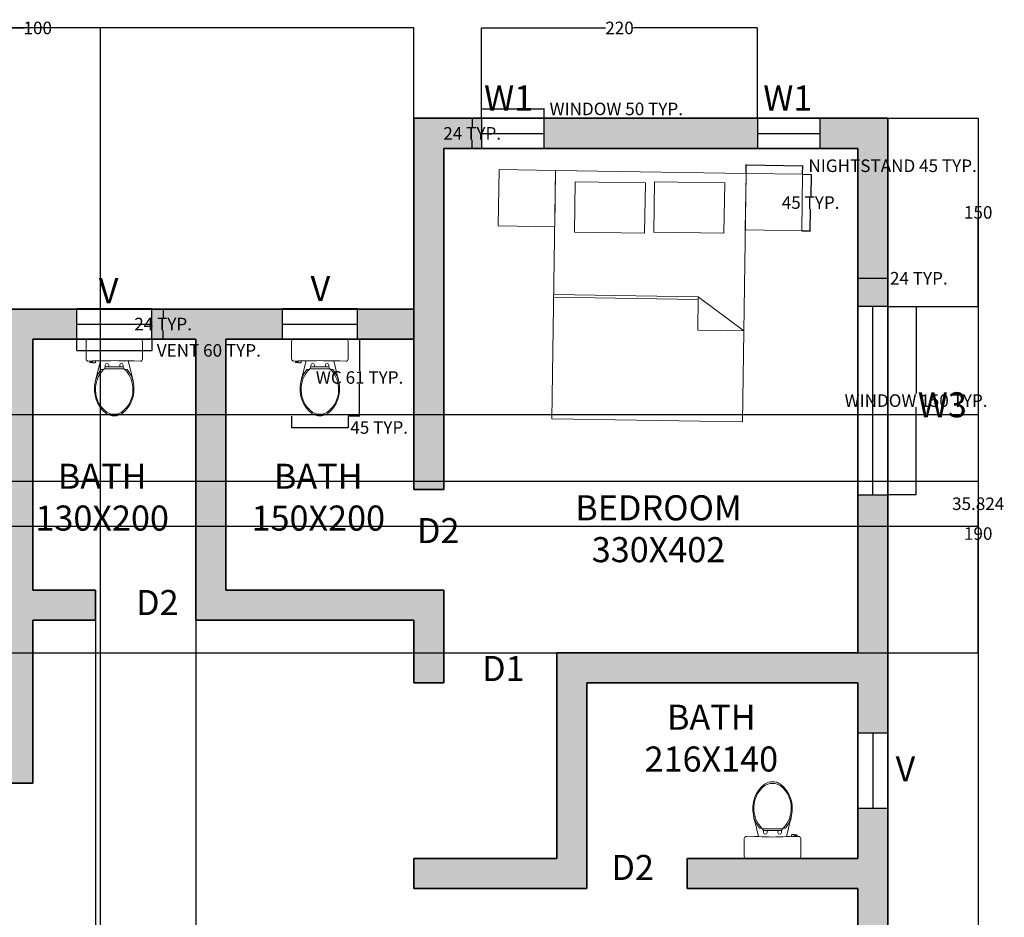
# Model space of a CAD drawing. Units: centimetres. Extents: x 1399 to 2860, y -110 to 1386.
# Tile 3 of 3: x 2074 to 2860, y 670 to 1386. Entities that reach past the tile are written whole.
import ezdxf

# ---------------------------------------------------------------- set-up
doc = ezdxf.new("R2010")
doc.units = ezdxf.units.CM
doc.header["$MEASUREMENT"] = 0
for name, color, linetype, lineweight in [('A-ANNO-DIMS', 2, 'Continuous', 18), ('A-ANNO-TEXT', 7, 'Continuous', 18), ('A-AREA-IDEN', 7, 'Continuous', 25), ('A-FLOR-FIXT', 9, 'Continuous', 18), ('A-FURN', 8, 'Continuous', 18), ('A-GLAZ', 4, 'Continuous', 25), ('A-WALL', 7, 'Continuous', 35), ('A-WALL-PATT', 252, 'Continuous', 13)]:
    doc.layers.add(name, color=color, linetype=linetype, lineweight=lineweight)
doc.styles.get("Standard").update_dxf_attribs({"font": 'arial.ttf'})
doc.dimstyles.get("Standard").update_dxf_attribs({"dimtxt": 10, "dimasz": 0.18, "dimexe": 0.18, "dimexo": 0.0625, "dimgap": 0.09, "dimtad": 0, "dimtih": 1, "dimtoh": 1, "dimdec": 4, "dimzin": 0, "dimdsep": 46, "dimtxsty": 'Standard', "dimcen": 0.09, "dimadec": 0, "dimazin": 0, "dimtfac": 1, "dimtdec": 4, "dimtofl": 0, "dimtmove": 0, "dimatfit": 3, "dimfxl": 1, "dimtolj": 1, "dimtzin": 0, "dimarcsym": 0})

# ---------------------------------------------------------------- blocks, each defined once
blk = doc.blocks.new('v')
blk.add_line((1187.13, 1404.19), (1237.13, 1404.19))
blk.add_lwpolyline([(1187.13, 1392.19), (1237.13, 1392.19), (1237.13, 1416.19), (1187.13, 1416.19)], close=True)
blk = doc.blocks.new('w1')
blk.add_line((1184.44, 1372.96), (1244.44, 1372.96))
blk.add_lwpolyline([(1184.44, 1360.96), (1244.44, 1360.96), (1244.44, 1384.96), (1184.44, 1384.96)], close=True)
blk = doc.blocks.new('w3')
blk.add_line((1235.35, 1319.41), (1085.35, 1319.41))
blk.add_lwpolyline([(1085.35, 1307.41), (1235.35, 1307.41), (1235.35, 1331.41), (1085.35, 1331.41)], close=True)
blk = doc.blocks.new('t')
for p, q in [((1419.3, 1723.8), (1428.5, 1740.5)), ((1428.5, 1740.5), (1428.5, 1758.8)), ((1461.3, 1740.5), (1428.5, 1740.5)), ((1461.3, 1758.8), (1461.3, 1740.5)), ((1513.8, 1740.5), (1461.3, 1740.5)), ((1513.8, 1740.5), (1566.3, 1740.5)), ((1566.3, 1758.8), (1566.3, 1740.5)), ((1566.3, 1740.5), (1599.1, 1740.5)), ((1599.1, 1740.5), (1599.1, 1758.8)), ((1608.3, 1723.8), (1599.1, 1740.5))]:
    blk.add_line(p, q)
for points in [[(1305.4, 1797.9), (1266, 1796.3, -0.426005), (1244, 1817.4), (1244, 1986.1, -0.414214), (1265.2, 2007.3), (1513.9, 2007.3)], [(1646.4, 1798.6, 0.00511), (1705.4, 1798.8), (1761.8, 1796.3, 0.426005), (1783.8, 1817.4), (1783.8, 1986.1, 0.414214), (1762.6, 2007.3), (1513.9, 2007.3)], [(1305.4, 1782.1), (1283.1, 1782.1, -0.3351), (1280.9, 1783.8), (1279.4, 1789.1, -0.498015), (1280.9, 1791.1), (1305.4, 1791.1)], [(1333.4, 1798.7), (1305.4, 1797.9, -0.319616)], [(1305.4, 1782.1), (1305.4, 1781.4, 0.414214), (1307.7, 1779.1), (1326.6, 1779.1, 0.414214), (1333.4, 1786), (1333.4, 1798.7)], [(1381.5, 1798.6, -0.006773), (1336.9, 1798.8), (1333.4, 1798.7, -0.55454)], [(1513.6, 1802.1, -0.010344), (1381.5, 1798.6)], [(1514.2, 1802.1, 0.010344), (1646.4, 1798.6)], [(1389.6, 1716.9, 0.114632), (1331.2, 1595.2, 0.16845)], [(1412.4, 1716.9, 0.434217), (1428.5, 1319.8, 0.182634), (1513.8, 1288.7, 2.693815)], [(1412.4, 1716.9), (1389.6, 1716.9, 0.416606)], [(1419.3, 1723.8, 0.008985), (1412.4, 1716.9, 0.182634)], [(1513.8, 1723.8), (1419.3, 1723.8, 0.008985)], [(1513.8, 1723.8), (1608.3, 1723.8, -0.444938)], [(1615.2, 1716.9, -0.434217), (1599.1, 1319.8, -0.182634), (1513.8, 1288.7, -2.693815)], [(1608.3, 1723.8, -0.008985), (1615.2, 1716.9, -0.182634)], [(1615.2, 1716.9), (1638, 1716.9, -0.416606)], [(1638, 1716.9, -0.117999), (1697.2, 1591.4, -0.16845)], [(1340.4, 1636.4, 0.005151), (1338.9, 1631, 0.024565), (1331.2, 1595.2, 0.065413)], [(1697.2, 1591.4, 0.0272), (1688.9, 1631, 0.005151), (1687.4, 1636.4, 0.103607)], [(1331.2, 1595.2, 0.288211), (1437.6, 1296.1, 0.171216), (1513.8, 1274, 2.912232)], [(1697.2, 1591.4, -0.284616), (1590, 1296.1, -0.171216), (1513.8, 1274, -2.912347)]]:
    blk.add_lwpolyline(points, format="xyb")
for points in [[(1305.4, 1797.9), (1305.4, 1791.1)], [(1305.4, 1791.1), (1305.4, 1782.1)], [(1340.4, 1636.4), (1381.5, 1798.6)], [(1687.4, 1636.4), (1646.4, 1798.6)]]:
    blk.add_lwpolyline(points)
for centre in [(1444.9, 1758.8), (1582.7, 1758.8)]:
    blk.add_arc(centre, 16.4, 0, 180)
blk = doc.blocks.new('BED')
for p, q in [((1734.14, 2886.74), (1849.51, 2886.74)), ((1734.14, 2884.74), (1849.51, 2884.74)), ((1849.51, 2886.74), (1886.14, 2860.24)), ((1886.14, 2860.24), (1849.51, 2886.74)), ((1849.51, 2886.74), (1849.51, 2860.24)), ((1849.51, 2860.24), (1886.14, 2860.24))]:
    blk.add_line(p, q)
for points in [[(1734.14, 2787.74), (1886.14, 2787.74), (1886.14, 2985.74), (1734.14, 2985.74)], [(1749.96, 2936.84), (1805.89, 2936.84), (1805.89, 2977.01), (1749.96, 2977.01)], [(1813.22, 2937.77), (1869.15, 2937.77), (1869.15, 2977.94), (1813.22, 2977.94)]]:
    blk.add_lwpolyline(points, close=True)
blk = doc.blocks.new('NIGHTSTAND-450')
blk.add_lwpolyline([(0, 45), (0, 0), (45, 0), (45, 45)], close=True)
blk = doc.blocks.new('*D13')
at = {"layer": 'A-ANNO-DIMS', "color": 0, "lineweight": -2, "transparency": 16777216}
for p, q in [((2442.8, 1307.07), (2442.8, 1314.69)), ((2442.98, 1314.51), (2492.62, 1314.51)), ((2492.8, 1307.07), (2492.8, 1314.69)), ((2492.8, 1314.51), (2492.98, 1314.51))]:
    blk.add_line(p, q, dxfattribs=at)
at = {"layer": 'A-ANNO-DIMS', "color": 0, "transparency": 16777216}
for points in [[(2442.98, 1314.54), (2442.98, 1314.48), (2442.8, 1314.51)], [(2492.62, 1314.54), (2492.62, 1314.48), (2492.8, 1314.51)]]:
    blk.add_solid(points, dxfattribs=at)
at = {"layer": 'Defpoints', "color": 0, "transparency": 16777216}
for p in [(2492.8, 1314.51), (2442.8, 1307.01), (2492.8, 1307.01)]:
    blk.add_point(p, dxfattribs=at)
at = {"layer": 'A-ANNO-DIMS', "color": 0, "transparency": 16777216, "insert": (2550.2, 1314.51), "char_height": 10, "attachment_point": 5}
blk.add_mtext('\\A1;WINDOW 50 TYP.', dxfattribs=at)
blk = doc.blocks.new('*D14')
at = {"layer": 'A-ANNO-DIMS', "color": 0, "lineweight": -2, "transparency": 16777216}
for p, q in [((2442.74, 1307.01), (2435.12, 1307.01)), ((2435.3, 1306.83), (2435.3, 1300.12)), ((2435.3, 1283.19), (2435.3, 1289.9)), ((2442.74, 1283.01), (2435.12, 1283.01))]:
    blk.add_line(p, q, dxfattribs=at)
at = {"layer": 'A-ANNO-DIMS', "color": 0, "transparency": 16777216}
for points in [[(2435.27, 1306.83), (2435.33, 1306.83), (2435.3, 1307.01)], [(2435.27, 1283.19), (2435.33, 1283.19), (2435.3, 1283.01)]]:
    blk.add_solid(points, dxfattribs=at)
at = {"layer": 'Defpoints', "color": 0, "transparency": 16777216}
for p in [(2435.3, 1307.01), (2442.8, 1307.01), (2442.8, 1283.01)]:
    blk.add_point(p, dxfattribs=at)
at = {"layer": 'A-ANNO-DIMS', "color": 0, "transparency": 16777216, "insert": (2435.3, 1295.01), "char_height": 10, "attachment_point": 5}
blk.add_mtext('\\A1;24 TYP.', dxfattribs=at)
blk = doc.blocks.new('*D15')
at = {"layer": 'A-ANNO-DIMS', "color": 0, "lineweight": -2, "transparency": 16777216}
for p, q in [((2766.86, 1157.01), (2789.48, 1157.01)), ((2789.3, 1156.83), (2789.3, 1087.27)), ((2789.3, 1007.19), (2789.3, 1076.75)), ((2766.86, 1007.01), (2789.48, 1007.01))]:
    blk.add_line(p, q, dxfattribs=at)
at = {"layer": 'A-ANNO-DIMS', "color": 0, "transparency": 16777216}
for points in [[(2789.27, 1156.83), (2789.33, 1156.83), (2789.3, 1157.01)], [(2789.27, 1007.19), (2789.33, 1007.19), (2789.3, 1007.01)]]:
    blk.add_solid(points, dxfattribs=at)
at = {"layer": 'Defpoints', "color": 0, "transparency": 16777216}
for p in [(2766.8, 1157.01), (2766.8, 1007.01), (2789.3, 1007.01)]:
    blk.add_point(p, dxfattribs=at)
at = {"layer": 'A-ANNO-DIMS', "color": 0, "transparency": 16777216, "insert": (2789.3, 1082.01), "char_height": 10, "attachment_point": 5}
blk.add_mtext('\\A1;WINDOW 150 TYP.', dxfattribs=at)
blk = doc.blocks.new('*D16')
at = {"layer": 'A-ANNO-DIMS', "color": 0, "lineweight": -2, "transparency": 16777216}
for p, q in [((2742.8, 1157.07), (2742.8, 1179.69)), ((2742.98, 1179.51), (2766.62, 1179.51)), ((2766.8, 1157.07), (2766.8, 1179.69)), ((2766.8, 1179.51), (2766.98, 1179.51))]:
    blk.add_line(p, q, dxfattribs=at)
at = {"layer": 'A-ANNO-DIMS', "color": 0, "transparency": 16777216}
for points in [[(2742.98, 1179.54), (2742.98, 1179.48), (2742.8, 1179.51)], [(2766.62, 1179.54), (2766.62, 1179.48), (2766.8, 1179.51)]]:
    blk.add_solid(points, dxfattribs=at)
at = {"layer": 'Defpoints', "color": 0, "transparency": 16777216}
for p in [(2766.8, 1179.51), (2742.8, 1157.01), (2766.8, 1157.01)]:
    blk.add_point(p, dxfattribs=at)
at = {"layer": 'A-ANNO-DIMS', "color": 0, "transparency": 16777216, "insert": (2791.5, 1179.51), "char_height": 10, "attachment_point": 5}
blk.add_mtext('\\A1;24 TYP.', dxfattribs=at)
blk = doc.blocks.new('*D17')
at = {"layer": 'A-ANNO-DIMS', "color": 0, "lineweight": -2, "transparency": 16777216}
for p, q in [((2119.8, 1130.95), (2119.8, 1121.83)), ((2179.8, 1130.95), (2179.8, 1121.83)), ((2119.98, 1122.01), (2179.62, 1122.01)), ((2179.8, 1122.01), (2179.98, 1122.01))]:
    blk.add_line(p, q, dxfattribs=at)
at = {"layer": 'A-ANNO-DIMS', "color": 0, "transparency": 16777216}
for points in [[(2119.98, 1122.04), (2119.98, 1121.98), (2119.8, 1122.01)], [(2179.62, 1122.04), (2179.62, 1121.98), (2179.8, 1122.01)]]:
    blk.add_solid(points, dxfattribs=at)
at = {"layer": 'Defpoints', "color": 0, "transparency": 16777216}
for p in [(2119.8, 1131.01), (2179.8, 1131.01), (2179.8, 1122.01)]:
    blk.add_point(p, dxfattribs=at)
at = {"layer": 'A-ANNO-DIMS', "color": 0, "transparency": 16777216, "insert": (2225.24, 1122.01), "char_height": 10, "attachment_point": 5}
blk.add_mtext('\\A1;VENT 60 TYP.', dxfattribs=at)
blk = doc.blocks.new('*D18')
at = {"layer": 'A-ANNO-DIMS', "color": 0, "lineweight": -2, "transparency": 16777216}
for p, q in [((2179.86, 1155.01), (2188.98, 1155.01)), ((2188.8, 1154.83), (2188.8, 1148.12)), ((2179.86, 1131.01), (2188.98, 1131.01)), ((2188.8, 1131.19), (2188.8, 1137.9))]:
    blk.add_line(p, q, dxfattribs=at)
at = {"layer": 'A-ANNO-DIMS', "color": 0, "transparency": 16777216}
for points in [[(2188.77, 1154.83), (2188.83, 1154.83), (2188.8, 1155.01)], [(2188.77, 1131.19), (2188.83, 1131.19), (2188.8, 1131.01)]]:
    blk.add_solid(points, dxfattribs=at)
at = {"layer": 'Defpoints', "color": 0, "transparency": 16777216}
for p in [(2179.8, 1155.01), (2188.8, 1155.01), (2179.8, 1131.01)]:
    blk.add_point(p, dxfattribs=at)
at = {"layer": 'A-ANNO-DIMS', "color": 0, "transparency": 16777216, "insert": (2188.8, 1143.01), "char_height": 10, "attachment_point": 5}
blk.add_mtext('\\A1;24 TYP.', dxfattribs=at)
blk = doc.blocks.new('*D25')
at = {"layer": 'A-ANNO-DIMS', "color": 0, "lineweight": -2, "transparency": 16777216}
for p, q in [((2653.79, 1263.2), (2653.9, 1270.07)), ((2654.08, 1269.88), (2698.71, 1269.2)), ((2698.79, 1262.51), (2698.89, 1269.37)), ((2698.89, 1269.19), (2699.07, 1269.19))]:
    blk.add_line(p, q, dxfattribs=at)
at = {"layer": 'A-ANNO-DIMS', "color": 0, "transparency": 16777216}
for points in [[(2654.08, 1269.91), (2654.08, 1269.85), (2653.9, 1269.89)], [(2698.71, 1269.23), (2698.71, 1269.17), (2698.89, 1269.19)]]:
    blk.add_solid(points, dxfattribs=at)
at = {"layer": 'Defpoints', "color": 0, "transparency": 16777216}
for p in [(2698.89, 1269.19), (2653.79, 1263.14), (2698.79, 1262.44)]:
    blk.add_point(p, dxfattribs=at)
at = {"layer": 'A-ANNO-DIMS', "color": 0, "transparency": 16777216, "insert": (2770.6, 1269.19), "char_height": 10, "attachment_point": 5}
blk.add_mtext('\\A1;NIGHTSTAND 45 TYP.', dxfattribs=at)
blk = doc.blocks.new('*D26')
at = {"layer": 'A-ANNO-DIMS', "color": 0, "lineweight": -2, "transparency": 16777216}
for p, q in [((2698.85, 1262.44), (2705.72, 1262.34)), ((2705.53, 1262.16), (2705.27, 1245.02)), ((2704.85, 1217.53), (2705.11, 1234.67)), ((2698.16, 1217.45), (2705.02, 1217.34))]:
    blk.add_line(p, q, dxfattribs=at)
at = {"layer": 'A-ANNO-DIMS', "color": 0, "transparency": 16777216}
for points in [[(2705.5, 1262.16), (2705.56, 1262.16), (2705.54, 1262.34)], [(2704.82, 1217.53), (2704.88, 1217.53), (2704.84, 1217.35)]]:
    blk.add_solid(points, dxfattribs=at)
at = {"layer": 'Defpoints', "color": 0, "transparency": 16777216}
for p in [(2698.79, 1262.44), (2698.1, 1217.45), (2704.84, 1217.35)]:
    blk.add_point(p, dxfattribs=at)
at = {"layer": 'A-ANNO-DIMS', "color": 0, "transparency": 16777216, "insert": (2705.19, 1239.84), "char_height": 10, "attachment_point": 5}
blk.add_mtext('\\A1;45 TYP.', dxfattribs=at)
blk = doc.blocks.new('*D27')
at = {"layer": 'A-ANNO-DIMS', "color": 0, "lineweight": -2, "transparency": 16777216}
for p, q in [((2336.36, 1131.01), (2345.66, 1131.01)), ((2345.48, 1130.83), (2345.48, 1105.65)), ((2345.48, 1069.96), (2345.48, 1095.13)), ((2336.36, 1069.78), (2345.66, 1069.78))]:
    blk.add_line(p, q, dxfattribs=at)
at = {"layer": 'A-ANNO-DIMS', "color": 0, "transparency": 16777216}
for points in [[(2345.45, 1130.83), (2345.51, 1130.83), (2345.48, 1131.01)], [(2345.45, 1069.96), (2345.51, 1069.96), (2345.48, 1069.78)]]:
    blk.add_solid(points, dxfattribs=at)
at = {"layer": 'Defpoints', "color": 0, "transparency": 16777216}
for p in [(2336.29, 1131.01), (2345.48, 1131.01), (2336.29, 1069.78)]:
    blk.add_point(p, dxfattribs=at)
at = {"layer": 'A-ANNO-DIMS', "color": 0, "transparency": 16777216, "insert": (2345.48, 1100.39), "char_height": 10, "attachment_point": 5}
blk.add_mtext('\\A1;WC 61 TYP.', dxfattribs=at)
blk = doc.blocks.new('*D28')
at = {"layer": 'A-ANNO-DIMS', "color": 0, "lineweight": -2, "transparency": 16777216}
for p, q in [((2291.31, 1069.71), (2291.31, 1060.41)), ((2336.29, 1069.71), (2336.29, 1060.41)), ((2291.49, 1060.59), (2336.11, 1060.59)), ((2336.29, 1060.59), (2336.47, 1060.59))]:
    blk.add_line(p, q, dxfattribs=at)
at = {"layer": 'A-ANNO-DIMS', "color": 0, "transparency": 16777216}
for points in [[(2291.49, 1060.62), (2291.49, 1060.56), (2291.31, 1060.59)], [(2336.11, 1060.62), (2336.11, 1060.56), (2336.29, 1060.59)]]:
    blk.add_solid(points, dxfattribs=at)
at = {"layer": 'Defpoints', "color": 0, "transparency": 16777216}
for p in [(2291.31, 1069.78), (2336.29, 1069.78), (2336.29, 1060.59)]:
    blk.add_point(p, dxfattribs=at)
at = {"layer": 'A-ANNO-DIMS', "color": 0, "transparency": 16777216, "insert": (2361.1, 1060.59), "char_height": 10, "attachment_point": 5}
blk.add_mtext('\\A1;45 TYP.', dxfattribs=at)
blk = doc.blocks.new('*D37')
at = {"layer": 'A-ANNO-DIMS', "color": 0, "lineweight": -2, "transparency": 16777216}
for p, q in [((1482.8, 800.95), (1482.8, -103.22)), ((2766.8, -31.05), (2766.8, -103.22)), ((1482.98, -103.04), (2110.27, -103.04)), ((2766.62, -103.04), (2139.33, -103.04))]:
    blk.add_line(p, q, dxfattribs=at)
at = {"layer": 'A-ANNO-DIMS', "color": 0, "transparency": 16777216}
for points in [[(1482.98, -103.01), (1482.98, -103.07), (1482.8, -103.04)], [(2766.62, -103.01), (2766.62, -103.07), (2766.8, -103.04)]]:
    blk.add_solid(points, dxfattribs=at)
at = {"layer": 'Defpoints', "color": 0, "transparency": 16777216}
for p in [(1482.8, 801.01), (2766.8, -30.99), (2766.8, -103.04)]:
    blk.add_point(p, dxfattribs=at)
at = {"layer": 'A-ANNO-DIMS', "color": 0, "transparency": 16777216, "insert": (2124.8, -103.04), "char_height": 10, "attachment_point": 5}
blk.add_mtext('\\A1;1284', dxfattribs=at)
blk = doc.blocks.new('*D38')
at = {"layer": 'A-ANNO-DIMS', "color": 0, "lineweight": -2, "transparency": 16777216}
for p, q in [((2766.86, 1307.01), (2839.03, 1307.01)), ((2838.85, 1306.83), (2838.85, 643.21)), ((2838.85, -30.81), (2838.85, 632.81)), ((2766.86, -30.99), (2839.03, -30.99))]:
    blk.add_line(p, q, dxfattribs=at)
at = {"layer": 'A-ANNO-DIMS', "color": 0, "transparency": 16777216}
for points in [[(2838.82, 1306.83), (2838.88, 1306.83), (2838.85, 1307.01)], [(2838.82, -30.81), (2838.88, -30.81), (2838.85, -30.99)]]:
    blk.add_solid(points, dxfattribs=at)
at = {"layer": 'Defpoints', "color": 0, "transparency": 16777216}
for p in [(2766.8, 1307.01), (2838.85, 1307.01), (2766.8, -30.99)]:
    blk.add_point(p, dxfattribs=at)
at = {"layer": 'A-ANNO-DIMS', "color": 0, "transparency": 16777216, "insert": (2838.85, 638.01), "char_height": 10, "attachment_point": 5}
blk.add_mtext('\\A1;1338', dxfattribs=at)
blk = doc.blocks.new('*D39')
at = {"layer": 'A-ANNO-DIMS', "color": 0, "lineweight": -2, "transparency": 16777216}
for p, q in [((1532.8, 1155.07), (1532.8, 1379.24)), ((1532.98, 1379.06), (1949.66, 1379.06)), ((2388.62, 1379.06), (1971.94, 1379.06)), ((2388.8, 1155.07), (2388.8, 1379.24))]:
    blk.add_line(p, q, dxfattribs=at)
at = {"layer": 'A-ANNO-DIMS', "color": 0, "transparency": 16777216}
for points in [[(1532.98, 1379.09), (1532.98, 1379.03), (1532.8, 1379.06)], [(2388.62, 1379.09), (2388.62, 1379.03), (2388.8, 1379.06)]]:
    blk.add_solid(points, dxfattribs=at)
at = {"layer": 'Defpoints', "color": 0, "transparency": 16777216}
for p in [(2388.8, 1379.06), (1532.8, 1155.01), (2388.8, 1155.01)]:
    blk.add_point(p, dxfattribs=at)
at = {"layer": 'A-ANNO-DIMS', "color": 0, "transparency": 16777216, "insert": (1960.8, 1379.06), "char_height": 10, "attachment_point": 5}
blk.add_mtext('\\A1;856', dxfattribs=at)
blk = doc.blocks.new('*D44')
at = {"layer": 'A-ANNO-DIMS', "color": 0, "lineweight": -2, "transparency": 16777216}
for p, q in [((2134.8, 906.95), (2134.8, -103.22)), ((2214.8, 906.95), (2214.8, -103.22)), ((2134.98, -103.04), (2167.56, -103.04)), ((2214.62, -103.04), (2182.04, -103.04))]:
    blk.add_line(p, q, dxfattribs=at)
at = {"layer": 'A-ANNO-DIMS', "color": 0, "transparency": 16777216}
for points in [[(2134.98, -103.01), (2134.98, -103.07), (2134.8, -103.04)], [(2214.62, -103.01), (2214.62, -103.07), (2214.8, -103.04)]]:
    blk.add_solid(points, dxfattribs=at)
at = {"layer": 'Defpoints', "color": 0, "transparency": 16777216}
for p in [(2134.8, 907.01), (2214.8, 907.01), (2214.8, -103.04)]:
    blk.add_point(p, dxfattribs=at)
at = {"layer": 'A-ANNO-DIMS', "color": 0, "transparency": 16777216, "insert": (2174.8, -103.04), "char_height": 10, "attachment_point": 5}
blk.add_mtext('\\A1;80', dxfattribs=at)
blk = doc.blocks.new('*D45')
at = {"layer": 'A-ANNO-DIMS', "color": 0, "lineweight": -2, "transparency": 16777216}
for p, q in [((2038.8, 33.07), (2038.8, 1379.24)), ((2038.98, 1379.06), (2078.15, 1379.06)), ((2138.62, 1379.06), (2099.45, 1379.06)), ((2138.8, 183.07), (2138.8, 1379.24))]:
    blk.add_line(p, q, dxfattribs=at)
at = {"layer": 'A-ANNO-DIMS', "color": 0, "transparency": 16777216}
for points in [[(2038.98, 1379.09), (2038.98, 1379.03), (2038.8, 1379.06)], [(2138.62, 1379.09), (2138.62, 1379.03), (2138.8, 1379.06)]]:
    blk.add_solid(points, dxfattribs=at)
at = {"layer": 'Defpoints', "color": 0, "transparency": 16777216}
for p in [(2038.8, 1379.06), (2138.8, 183.01), (2038.8, 33.01)]:
    blk.add_point(p, dxfattribs=at)
at = {"layer": 'A-ANNO-DIMS', "color": 0, "transparency": 16777216, "insert": (2088.8, 1379.06), "char_height": 10, "attachment_point": 5}
blk.add_mtext('\\A1;100', dxfattribs=at)
blk = doc.blocks.new('*D46')
at = {"layer": 'A-ANNO-DIMS', "color": 0, "lineweight": -2, "transparency": 16777216}
for p, q in [((2442.8, 1307.07), (2442.8, 1379.24)), ((2442.98, 1379.06), (2541.6, 1379.06)), ((2662.62, 1379.06), (2564.01, 1379.06)), ((2662.8, 1307.07), (2662.8, 1379.24))]:
    blk.add_line(p, q, dxfattribs=at)
at = {"layer": 'A-ANNO-DIMS', "color": 0, "transparency": 16777216}
for points in [[(2442.98, 1379.09), (2442.98, 1379.03), (2442.8, 1379.06)], [(2662.62, 1379.09), (2662.62, 1379.03), (2662.8, 1379.06)]]:
    blk.add_solid(points, dxfattribs=at)
at = {"layer": 'Defpoints', "color": 0, "transparency": 16777216}
for p in [(2662.8, 1379.06), (2442.8, 1307.01), (2662.8, 1307.01)]:
    blk.add_point(p, dxfattribs=at)
at = {"layer": 'A-ANNO-DIMS', "color": 0, "transparency": 16777216, "insert": (2552.8, 1379.06), "char_height": 10, "attachment_point": 5}
blk.add_mtext('\\A1;220', dxfattribs=at)
blk = doc.blocks.new('*D47')
at = {"layer": 'A-ANNO-DIMS', "color": 0, "lineweight": -2, "transparency": 16777216}
for p, q in [((2766.86, 1307.01), (2839.03, 1307.01)), ((2838.85, 1306.83), (2838.85, 1237.21)), ((2838.85, 1157.19), (2838.85, 1226.81)), ((2766.86, 1157.01), (2839.03, 1157.01))]:
    blk.add_line(p, q, dxfattribs=at)
at = {"layer": 'A-ANNO-DIMS', "color": 0, "transparency": 16777216}
for points in [[(2838.82, 1306.83), (2838.88, 1306.83), (2838.85, 1307.01)], [(2838.82, 1157.19), (2838.88, 1157.19), (2838.85, 1157.01)]]:
    blk.add_solid(points, dxfattribs=at)
at = {"layer": 'Defpoints', "color": 0, "transparency": 16777216}
for p in [(2766.8, 1307.01), (2838.85, 1307.01), (2766.8, 1157.01)]:
    blk.add_point(p, dxfattribs=at)
at = {"layer": 'A-ANNO-DIMS', "color": 0, "transparency": 16777216, "insert": (2838.85, 1232.01), "char_height": 10, "attachment_point": 5}
blk.add_mtext('\\A1;150', dxfattribs=at)
blk = doc.blocks.new('*D51')
at = {"layer": 'A-ANNO-DIMS', "color": 0, "lineweight": -2, "transparency": 16777216}
for p, q in [((1600.97, 1017.69), (2839.03, 1017.69)), ((2838.85, 1017.51), (2838.85, 1004.98)), ((2838.85, 982.05), (2838.85, 994.58)), ((1600.97, 981.87), (2839.03, 981.87))]:
    blk.add_line(p, q, dxfattribs=at)
at = {"layer": 'A-ANNO-DIMS', "color": 0, "transparency": 16777216}
for points in [[(2838.82, 1017.51), (2838.88, 1017.51), (2838.85, 1017.69)], [(2838.82, 982.05), (2838.88, 982.05), (2838.85, 981.87)]]:
    blk.add_solid(points, dxfattribs=at)
at = {"layer": 'Defpoints', "color": 0, "transparency": 16777216}
for p in [(1600.91, 1017.69), (1600.91, 981.87), (2838.85, 981.87)]:
    blk.add_point(p, dxfattribs=at)
at = {"layer": 'A-ANNO-DIMS', "color": 0, "transparency": 16777216, "insert": (2838.85, 999.78), "char_height": 10, "attachment_point": 5}
blk.add_mtext('\\A1;35.824', dxfattribs=at)
blk = doc.blocks.new('*D53')
at = {"layer": 'A-ANNO-DIMS', "color": 0, "lineweight": -2, "transparency": 16777216}
for p, q in [((1790.86, 1071.01), (2839.03, 1071.01)), ((2838.85, 1070.83), (2838.85, 981.21)), ((2838.85, 881.19), (2838.85, 970.81)), ((1790.86, 881.01), (2839.03, 881.01))]:
    blk.add_line(p, q, dxfattribs=at)
at = {"layer": 'A-ANNO-DIMS', "color": 0, "transparency": 16777216}
for points in [[(2838.82, 1070.83), (2838.88, 1070.83), (2838.85, 1071.01)], [(2838.82, 881.19), (2838.88, 881.19), (2838.85, 881.01)]]:
    blk.add_solid(points, dxfattribs=at)
at = {"layer": 'Defpoints', "color": 0, "transparency": 16777216}
for p in [(1790.8, 1071.01), (2838.85, 1071.01), (1790.8, 881.01)]:
    blk.add_point(p, dxfattribs=at)
at = {"layer": 'A-ANNO-DIMS', "color": 0, "transparency": 16777216, "insert": (2838.85, 976.01), "char_height": 10, "attachment_point": 5}
blk.add_mtext('\\A1;190', dxfattribs=at)

msp = doc.modelspace()

# ---------------------------------------------------------------- hatches: boundary and pattern name
at = {"layer": 'A-WALL-PATT'}
h = msp.add_hatch(color=256, dxfattribs=at)
h.dxf.hatch_style = 1
h.paths.add_polyline_path([(1581.8022, 1155.0098), (1532.8022, 1155.0098), (1532.8022, 1081.0098), (1556.8022, 1081.0098), (1556.8022, 1131.0098), (1581.8022, 1131.0098)])
h.paths.add_polyline_path([(1556.8022, 931.0098), (1532.8022, 931.0098), (1532.8022, 881.0098), (1556.8022, 881.0098)])
h.paths.add_polyline_path([(1820.8022, 1155.0098), (1681.8022, 1155.0098), (1681.8022, 1131.0098), (1706.8022, 1131.0098), (1706.8022, 881.0098), (1730.8022, 881.0098), (1730.8022, 1131.0098), (1820.8022, 1131.0098)])
h.paths.add_polyline_path([(2119.8022, 1155.0098), (1970.8022, 1155.0098), (1970.8022, 1131.0098), (2060.8022, 1131.0098), (2060.8022, 777.0098), (2084.8022, 777.0098), (2084.8022, 907.0098), (2134.8022, 907.0098), (2134.8022, 931.0098), (2084.8022, 931.0098), (2084.8022, 1131.0098), (2119.8022, 1131.0098)])
h.paths.add_polyline_path([(2283.8022, 1155.0098), (2179.8022, 1155.0098), (2179.8022, 1131.0098), (2214.8022, 1131.0098), (2214.8022, 907.0098), (2388.8022, 907.0098), (2388.8022, 857.0098), (2412.8022, 857.0098), (2412.8022, 931.0098), (2238.8022, 931.0098), (2238.8022, 1131.0098), (2283.8022, 1131.0098)])
h.paths.add_polyline_path([(2388.8022, 1155.0098), (2343.8022, 1155.0098), (2343.8022, 1131.0098), (2388.8022, 1131.0098)], flags=17)
h.paths.add_polyline_path([(2412.8022, 1283.0098), (2442.8022, 1283.0098), (2442.8022, 1307.0098), (2388.8022, 1307.0098), (2388.8022, 1011.0098), (2412.8022, 1011.0098)])
h.paths.add_polyline_path([(2662.8022, 1307.0098), (2492.8022, 1307.0098), (2492.8022, 1283.0098), (2662.8022, 1283.0098)])
h.paths.add_polyline_path([(2766.8022, 1307.0098), (2712.8022, 1307.0098), (2712.8022, 1283.0098), (2742.8022, 1283.0098), (2742.8022, 1157.0098), (2766.8022, 1157.0098)])
h.paths.add_polyline_path([(2766.8022, 1007.0098), (2742.8022, 1007.0098), (2742.8022, 881.0098), (2502.8022, 881.0098), (2502.8022, 717.0098), (2388.8022, 717.0098), (2388.8022, 693.0098), (2526.8022, 693.0098), (2526.8022, 857.0098), (2742.8022, 857.0098), (2742.8022, 817.0098), (2766.8022, 817.0098)])
h.paths.add_polyline_path([(2766.8022, 757.0098), (2742.8022, 757.0098), (2742.8022, 717.0098), (2606.8022, 717.0098), (2606.8022, 693.0098), (2742.8022, 693.0098), (2742.8022, 598.0098), (2766.8022, 598.0098)])
h.paths.add_polyline_path([(2442.8022, 353.0098), (2412.8022, 353.0098), (2412.8022, 603.0098), (2238.8022, 603.0098), (2238.8022, 579.0098), (2388.8022, 579.0098), (2388.8022, 512.2445, -0.02916898), (2388.8858, 510.8126), (2388.8858, 458.2748), (2388.8022, 458.2748), (2388.8022, 402.9002), (2388.8024, 402.776), (2388.8858, 402.776), (2388.8858, 350.2798, -0.02916898), (2388.8022, 348.8479), (2388.8022, 329.0098), (2442.8022, 329.0098)])
h.paths.add_polyline_path([(2662.8022, 353.0098), (2492.8022, 353.0098), (2492.8022, 329.0098), (2662.8022, 329.0098)])
h.paths.add_polyline_path([(2412.8022, 329.0098), (2388.8022, 329.0098), (2388.8022, 159.0098), (2412.8022, 159.0098)])
h.paths.add_polyline_path([(2388.8022, 183.0098), (2338.8022, 183.0098), (2338.8022, 159.0098), (2388.8022, 159.0098)])
h.paths.add_polyline_path([(2188.8022, 183.0098), (2138.8022, 183.0098), (2138.8022, 159.0098), (2188.8022, 159.0098)])
h.paths.add_polyline_path([(2038.8022, 417.0098), (2014.8022, 417.0098), (2014.8022, 33.0098), (1924.8022, 33.0098), (1924.8022, 9.0098), (2038.8022, 9.0098)])
h.paths.add_polyline_path([(1774.8022, 33.0098), (1684.8022, 33.0098), (1684.8022, 63.0098), (1660.8022, 63.0098), (1660.8022, 9.0098), (1774.8022, 9.0098)])
h.paths.add_polyline_path([(1684.8022, 313.0098), (1660.8022, 313.0098), (1660.8022, 113.0098), (1684.8022, 113.0098)])
h.paths.add_polyline_path([(1924.8022, 417.0098), (1684.8022, 417.0098), (1684.8022, 497.0098), (1660.8022, 497.0098), (1660.8022, 363.0098), (1684.8022, 363.0098), (1684.8022, 393.0098), (1924.8022, 393.0098)])
h.paths.add_polyline_path([(1684.8022, 777.0098), (1660.8022, 777.0098), (1660.8022, 697.0098), (1684.8022, 697.0098)])
h.paths.add_polyline_path([(1970.8022, 801.0098), (1532.8022, 801.0098), (1532.8022, 777.0098), (1970.8022, 777.0098)])

# ---------------------------------------------------------------- linework, layer by layer
at = {"layer": 'A-WALL'}
for p, q in [((2388.8022, 1307.0098), (2766.8022, 1307.0098)), ((2388.8022, 1011.0098), (2388.8022, 1307.0098)), ((2766.8022, -30.9902), (2766.8022, 1307.0098)), ((2412.8022, 1283.0098), (2742.8022, 1283.0098)), ((2412.8022, 1011.0098), (2412.8022, 1283.0098)), ((2742.8022, 881.0098), (2742.8022, 1283.0098)), ((1532.8022, 1155.0098), (2388.8022, 1155.0098)), ((2084.8022, 1131.0098), (2214.8022, 1131.0098)), ((2084.8022, 931.0098), (2084.8022, 1131.0098)), ((2214.8022, 907.0098), (2214.8022, 1131.0098)), ((2238.8022, 931.0098), (2238.8022, 1131.0098)), ((2238.8022, 1131.0098), (2388.8022, 1131.0098)), ((2388.8022, 1011.0098), (2412.8022, 1011.0098)), ((2084.8022, 931.0098), (2134.8022, 931.0098)), ((2134.8022, 907.0098), (2134.8022, 931.0098)), ((2238.8022, 931.0098), (2412.8022, 931.0098)), ((2412.8022, 857.0098), (2412.8022, 931.0098)), ((2084.8022, 777.0098), (2084.8022, 907.0098)), ((2084.8022, 907.0098), (2134.8022, 907.0098)), ((2214.8022, 907.0098), (2388.8022, 907.0098)), ((2388.8022, 857.0098), (2388.8022, 907.0098)), ((2502.8022, 717.0098), (2502.8022, 881.0098)), ((2502.8022, 881.0098), (2742.8022, 881.0098)), ((2388.8022, 857.0098), (2412.8022, 857.0098)), ((2526.8022, 693.0098), (2526.8022, 857.0098)), ((2526.8022, 857.0098), (2742.8022, 857.0098)), ((2742.8022, 717.0098), (2742.8022, 857.0098)), ((2060.8022, 777.0098), (2084.8022, 777.0098)), ((2388.8022, 717.0098), (2502.8022, 717.0098)), ((2388.8022, 693.0098), (2388.8022, 717.0098)), ((2606.8022, 693.0098), (2606.8022, 717.0098)), ((2606.8022, 717.0098), (2742.8022, 717.0098)), ((2388.8022, 693.0098), (2526.8022, 693.0098)), ((2606.8022, 693.0098), (2742.8022, 693.0098)), ((2742.8022, 353.0098), (2742.8022, 693.0098))]:
    msp.add_line(p, q, dxfattribs=at)

# ---------------------------------------------------------------- block references
at = {"layer": 'A-FLOR-FIXT', "xscale": 0.0833333333333333, "yscale": 0.0833333333333333, "zscale": 0.0833333333333333}
for p in [(2023.6429, 963.7375), (2187.6429, 963.7375)]:
    msp.add_blockref('t', p, dxfattribs=at)
at = {"layer": 'A-FLOR-FIXT', "xscale": 0.0833333333333333, "yscale": 0.0833333333333333, "zscale": 0.0833333333333333, "rotation": 180}
msp.add_blockref('t', (2800.9615, 884.282), dxfattribs=at)
at = {"layer": 'A-FURN'}
for name, p, rotation in [('NIGHTSTAND-450', (2456.8165, 1266.17), 269.1178617061952), ('BED', (721.9098, -1693.2097), 359.1178617061952), ('NIGHTSTAND-450', (2653.7932, 1263.1371), 269.1178617061952)]:
    msp.add_blockref(name, p, dxfattribs=dict(at, rotation=rotation))
at = {"layer": 'A-GLAZ'}
for name, p in [('v', (1255.672, -109.1797)), ('v', (1475.672, -109.1797)), ('w1', (935.3655, -229.9466)), ('w1', (1099.3655, -229.9466))]:
    msp.add_blockref(name, p, dxfattribs=at)
at = {"layer": 'A-GLAZ', "rotation": 270}
for name, p in [('w3', (1435.392, 2242.3567)), ('w1', (1381.8458, 2001.4465))]:
    msp.add_blockref(name, p, dxfattribs=at)

# ---------------------------------------------------------------- texts
at = {"layer": 'A-ANNO-TEXT', "char_height": 20, "attachment_point": 1}
for s, width, insert in [('W1', 163.588182, (2444.7907, 1333.1968)), ('W1', 163.588182, (2667.4449, 1333.1968)), ('V', 163.588182, (2137.4692, 1179.6364)), ('V', 163.588182, (2306.3723, 1181.308)), ('W3', 163.588182, (2790.6959, 1088.6513)), ('D2', 163.588182, (2391.2723, 988.3825)), ('D2', 163.588182, (2167.2367, 931.0308)), ('D1', 103.726959, (2443.1948, 878.4317)), ('V', 163.588182, (2772.9464, 798.5152)), ('D2', 163.588182, (2546.3314, 719.8123))]:
    msp.add_mtext_dynamic_manual_height_columns(s, width=width, gutter_width=1, heights=[0], dxfattribs=dict(at, insert=insert))
at = {"layer": 'A-AREA-IDEN', "char_height": 20, "attachment_point": 1}
for s, insert in [('\\pxqc;BATH\\P130X200', (1906.8609, 1031.6996)), ('\\pxqc;BATH\\P150X200', (2079.2039, 1031.6996)), ('\\pxqc;BEDROOM\\P330X402', (2350.5729, 1006.5233)), ('\\pxqc;BATH\\P216X140', (2392.7005, 839.6268))]:
    msp.add_mtext_dynamic_manual_height_columns(s, width=466.660539, gutter_width=1, heights=[0], dxfattribs=dict(at, insert=insert))

# ---------------------------------------------------------------- dimensions: what is measured, and where the dimension line sits
at = {"layer": 'A-ANNO-DIMS'}
for base, p1, p2, picture, middle in [((2388.8022, 1379.0598), (1532.8022, 1155.0098), (2388.8022, 1155.0098), '*D39', (1960.8022, 1379.0598)), ((2038.8022, 1379.0598), (2138.8022, 183.0098), (2038.8022, 33.0098), '*D45', (2088.8022, 1379.0598)), ((2662.8022, 1379.0598), (2442.8022, 1307.0098), (2662.8022, 1307.0098), '*D46', (2552.8022, 1379.0598)), ((2214.8022, -103.0402), (2134.8022, 907.0098), (2214.8022, 907.0098), '*D44', (2174.8022, -103.0402)), ((2766.8022, -103.0402), (1482.8022, 801.0098), (2766.8022, -30.9902), '*D37', (2124.8022, -103.0402))]:
    dim = msp.add_linear_dim(base=base, p1=p1, p2=p2, dimstyle='Standard', override={"dimdec": 0, "dimlfac": 1, "dimrnd": 0, "dimzin": 0, "dimdsep": 46, "dimlunit": 2}, dxfattribs=at)
    dim.commit()
    dim.dimension.update_dxf_attribs({"geometry": picture, "text_midpoint": middle})
for base, p1, p2, text, picture, middle in [((2492.8022, 1314.5098), (2442.8022, 1307.0098), (2492.8022, 1307.0098), 'WINDOW <> TYP.', '*D13', (2550.2038, 1314.5098)), ((2766.8022, 1179.5098), (2742.8022, 1157.0098), (2766.8022, 1157.0098), '<> TYP.', '*D16', (2791.4958, 1179.5098)), ((2179.8022, 1122.0098), (2119.8022, 1131.0098), (2179.8022, 1131.0098), 'VENT <> TYP.', '*D17', (2225.2393, 1122.0098)), ((2336.2927, 1060.5899), (2291.3116, 1069.7751), (2336.2927, 1069.7751), '<> TYP.', '*D28', (2361.1023, 1060.5899))]:
    dim = msp.add_linear_dim(base=base, p1=p1, p2=p2, text=text, dimstyle='Standard', override={"dimdec": 0, "dimlfac": 1, "dimrnd": 0, "dimzin": 0, "dimdsep": 46, "dimlunit": 2}, dxfattribs=at)
    dim.commit()
    dim.dimension.update_dxf_attribs({"geometry": picture, "text_midpoint": middle})
for base, p1, p2, angle, text, picture, middle in [((2435.3022, 1307.0098), (2442.8022, 1283.0098), (2442.8022, 1307.0098), 90, '<> TYP.', '*D14', (2435.3022, 1295.0098)), ((2698.8918, 1269.1935), (2653.7932, 1263.1371), (2698.7878, 1262.4443), 359.1178617, 'NIGHTSTAND <> TYP.', '*D25', (2770.601, 1269.1907)), ((2704.8442, 1217.3457), (2698.7878, 1262.4443), (2698.095, 1217.4496), 269.1178617, '<> TYP.', '*D26', (2705.1906, 1239.843)), ((2188.8022, 1155.0098), (2179.8022, 1131.0098), (2179.8022, 1155.0098), 90, '<> TYP.', '*D18', (2188.8022, 1143.0098)), ((2789.3022, 1007.0098), (2766.8022, 1157.0098), (2766.8022, 1007.0098), 270, 'WINDOW <> TYP.', '*D15', (2789.3022, 1082.0098)), ((2345.4779, 1131.0098), (2336.2927, 1069.7751), (2336.2927, 1131.0098), 90, 'WC <> TYP.', '*D27', (2345.4779, 1100.3925))]:
    dim = msp.add_linear_dim(base=base, p1=p1, p2=p2, angle=angle, text=text, dimstyle='Standard', override={"dimdec": 0, "dimlfac": 1, "dimrnd": 0, "dimzin": 0, "dimdsep": 46, "dimlunit": 2}, dxfattribs=at)
    dim.commit()
    dim.dimension.update_dxf_attribs({"geometry": picture, "text_midpoint": middle})
for base, p1, p2, override, picture, middle in [((2838.8522, 1307.0098), (2766.8022, -30.9902), (2766.8022, 1307.0098), {"dimdec": 0, "dimlfac": 1, "dimrnd": 0, "dimzin": 0, "dimdsep": 46, "dimlunit": 2}, '*D38', (2838.8522, 638.0098)), ((2838.8522, 1307.0098), (2766.8022, 1157.0098), (2766.8022, 1307.0098), {"dimdec": 0, "dimlfac": 1, "dimrnd": 0, "dimzin": 0, "dimdsep": 46, "dimlunit": 2}, '*D47', (2838.8522, 1232.0098)), ((2838.8522, 1071.0098), (1790.8022, 881.0098), (1790.8022, 1071.0098), {"dimdec": 0, "dimlfac": 1, "dimrnd": 0, "dimzin": 0, "dimdsep": 46, "dimlunit": 2}, '*D53', (2838.8522, 976.0098)), ((2838.8522, 981.8663), (1600.9054, 1017.6901), (1600.9054, 981.8663), {"dimdec": 3, "dimlfac": 1, "dimrnd": 0, "dimzin": 0, "dimdsep": 46, "dimlunit": 2}, '*D51', (2838.8522, 999.7782))]:
    dim = msp.add_linear_dim(base=base, p1=p1, p2=p2, angle=90, dimstyle='Standard', override=override, dxfattribs=at)
    dim.commit()
    dim.dimension.update_dxf_attribs({"geometry": picture, "text_midpoint": middle})

doc.saveas('drawing.dxf')
